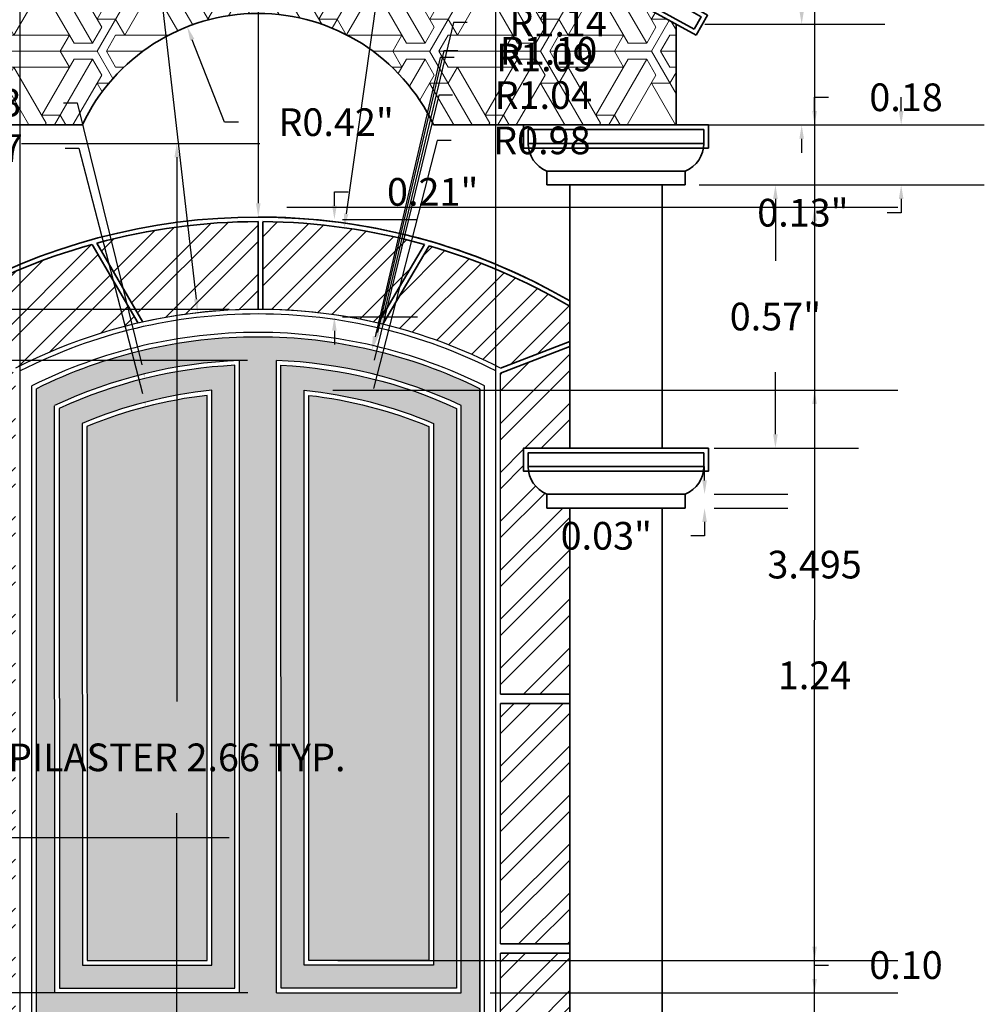
# Model space of a CAD drawing. Units: inches. Extents: x 19.36 to 24.97, y -1.46 to 4.09.
# Tile 3 of 4: x 20.47 to 22.56, y 0.85 to 2.98. Entities that reach past the tile are written whole.
import ezdxf

# ---------------------------------------------------------------- set-up
doc = ezdxf.new("R2010")
doc.units = ezdxf.units.IN
doc.header["$MEASUREMENT"] = 0
for name, color, linetype, lineweight in [('A-ANNO-DIMS', 2, 'Continuous', 18), ('A-COLS', 3, 'Continuous', 35), ('A-DOOR', 4, 'Continuous', 25), ('A-ELEV', 7, 'Continuous', 35), ('A-ELEV-PATT', 8, 'Continuous', 13)]:
    doc.layers.add(name, color=color, linetype=linetype, lineweight=lineweight)
doc.styles.get("Standard").update_dxf_attribs({"font": 'arial.ttf'})
doc.dimstyles.get("Standard").update_dxf_attribs({"dimtxt": 0.06, "dimasz": 0.03, "dimexe": 0.18, "dimexo": 0.0625, "dimgap": 0.09, "dimtad": 0, "dimtih": 1, "dimtoh": 1, "dimzin": 0, "dimdsep": 46, "dimlunit": 3, "dimtxsty": 'Standard', "dimcen": 0, "dimadec": 0, "dimazin": 0, "dimtfac": 1, "dimtofl": 0, "dimtmove": 0, "dimatfit": 3, "dimfxl": 1, "dimtolj": 1, "dimtzin": 0, "dimarcsym": 1})

# ---------------------------------------------------------------- blocks, each defined once
blk = doc.blocks.new('*D5')
at = {"layer": 'A-ANNO-DIMS', "color": 0, "lineweight": -2, "transparency": 16777216}
for p, q in [((21.1539, 2.5751), (21.1539, 2.6051)), ((21.1539, 2.6051), (21.1839, 2.6051)), ((21.1717, 2.5451), (21.3339, 2.5451)), ((21.1717, 2.3341), (21.3339, 2.3341)), ((21.1539, 2.3041), (21.1539, 2.2741))]:
    blk.add_line(p, q, dxfattribs=at)
at = {"layer": 'A-ANNO-DIMS', "color": 0, "transparency": 16777216}
for points in [[(21.1489, 2.5751), (21.1589, 2.5751), (21.1539, 2.5451)], [(21.1489, 2.3041), (21.1589, 2.3041), (21.1539, 2.3341)]]:
    blk.add_solid(points, dxfattribs=at)
at = {"layer": 'Defpoints', "color": 0, "transparency": 16777216}
for p in [(21.1092, 2.5451), (21.1539, 2.5451), (21.1092, 2.3341)]:
    blk.add_point(p, dxfattribs=at)
at = {"layer": 'A-ANNO-DIMS', "color": 0, "transparency": 16777216, "insert": (21.3667, 2.6051), "char_height": 0.06, "attachment_point": 5}
blk.add_mtext('\\A1;0.21"', dxfattribs=at)
blk = doc.blocks.new('*D6')
at = {"layer": 'A-ANNO-DIMS', "color": 0, "lineweight": -2, "transparency": 16777216}
for p, q in [((22.1656, 2.9981), (22.1656, 3.0281)), ((22.1656, 3.0281), (22.1956, 3.0281)), ((21.9561, 2.9681), (22.3456, 2.9681)), ((21.9561, 2.75), (22.3456, 2.75)), ((22.1656, 2.72), (22.1656, 2.69))]:
    blk.add_line(p, q, dxfattribs=at)
at = {"layer": 'A-ANNO-DIMS', "color": 0, "transparency": 16777216}
for points in [[(22.1606, 2.9981), (22.1706, 2.9981), (22.1656, 2.9681)], [(22.1606, 2.72), (22.1706, 2.72), (22.1656, 2.75)]]:
    blk.add_solid(points, dxfattribs=at)
at = {"layer": 'Defpoints', "color": 0, "transparency": 16777216}
for p in [(21.8936, 2.9681), (22.1656, 2.9681), (21.8936, 2.75)]:
    blk.add_point(p, dxfattribs=at)
at = {"layer": 'A-ANNO-DIMS', "color": 0, "transparency": 16777216, "insert": (22.3783, 3.0281), "char_height": 0.06, "attachment_point": 5}
blk.add_mtext('\\A1;0.22"', dxfattribs=at)
blk = doc.blocks.new('*D7')
at = {"layer": 'A-ANNO-DIMS', "color": 0, "lineweight": -2, "transparency": 16777216}
for p, q in [((22.381, 2.78), (22.381, 2.81)), ((21.9439, 2.75), (22.561, 2.75)), ((21.9439, 2.62), (22.561, 2.62)), ((22.381, 2.59), (22.381, 2.56)), ((22.381, 2.56), (22.351, 2.56))]:
    blk.add_line(p, q, dxfattribs=at)
at = {"layer": 'A-ANNO-DIMS', "color": 0, "transparency": 16777216}
for points in [[(22.376, 2.78), (22.386, 2.78), (22.381, 2.75)], [(22.376, 2.59), (22.386, 2.59), (22.381, 2.62)]]:
    blk.add_solid(points, dxfattribs=at)
at = {"layer": 'Defpoints', "color": 0, "transparency": 16777216}
for p in [(21.8814, 2.75), (21.8814, 2.62), (22.381, 2.62)]:
    blk.add_point(p, dxfattribs=at)
at = {"layer": 'A-ANNO-DIMS', "color": 0, "transparency": 16777216, "insert": (22.1683, 2.56), "char_height": 0.06, "attachment_point": 5}
blk.add_mtext('\\A1;0.13"', dxfattribs=at)
blk = doc.blocks.new('*D8')
at = {"layer": 'A-ANNO-DIMS', "color": 0, "lineweight": -2, "transparency": 16777216}
for p, q in [((21.9666, 2.62), (22.2888, 2.62)), ((22.1088, 2.59), (22.1088, 2.4556)), ((22.1088, 2.08), (22.1088, 2.2144)), ((21.9761, 2.05), (22.2888, 2.05))]:
    blk.add_line(p, q, dxfattribs=at)
at = {"layer": 'A-ANNO-DIMS', "color": 0, "transparency": 16777216}
for points in [[(22.1038, 2.59), (22.1138, 2.59), (22.1088, 2.62)], [(22.1038, 2.08), (22.1138, 2.08), (22.1088, 2.05)]]:
    blk.add_solid(points, dxfattribs=at)
at = {"layer": 'Defpoints', "color": 0, "transparency": 16777216}
for p in [(21.9041, 2.62), (21.9136, 2.05), (22.1088, 2.05)]:
    blk.add_point(p, dxfattribs=at)
at = {"layer": 'A-ANNO-DIMS', "color": 0, "transparency": 16777216, "insert": (22.1088, 2.335), "char_height": 0.06, "attachment_point": 5}
blk.add_mtext('\\A1;0.57"', dxfattribs=at)
blk = doc.blocks.new('*D9')
at = {"layer": 'A-ANNO-DIMS', "color": 0, "lineweight": -2, "transparency": 16777216}
for p, q in [((21.9554, 1.98), (21.9554, 2.01)), ((21.9761, 1.95), (22.1354, 1.95)), ((21.9761, 1.92), (22.1354, 1.92)), ((21.9554, 1.89), (21.9554, 1.86)), ((21.9554, 1.86), (21.9254, 1.86))]:
    blk.add_line(p, q, dxfattribs=at)
at = {"layer": 'A-ANNO-DIMS', "color": 0, "transparency": 16777216}
for points in [[(21.9504, 1.98), (21.9604, 1.98), (21.9554, 1.95)], [(21.9504, 1.89), (21.9604, 1.89), (21.9554, 1.92)]]:
    blk.add_solid(points, dxfattribs=at)
at = {"layer": 'Defpoints', "color": 0, "transparency": 16777216}
for p in [(21.9136, 1.95), (21.9136, 1.92), (21.9554, 1.92)]:
    blk.add_point(p, dxfattribs=at)
at = {"layer": 'A-ANNO-DIMS', "color": 0, "transparency": 16777216, "insert": (21.7426, 1.86), "char_height": 0.06, "attachment_point": 5}
blk.add_mtext('\\A1;0.03"', dxfattribs=at)
blk = doc.blocks.new('*D15')
at = {"layer": 'A-ANNO-DIMS', "color": 0, "lineweight": -2, "transparency": 16777216}
for p, q in [((20.9161, 2.7561), (20.8461, 2.9348)), ((20.9461, 2.7561), (20.9161, 2.7561))]:
    blk.add_line(p, q, dxfattribs=at)
at = {"layer": 'A-ANNO-DIMS', "color": 0, "transparency": 16777216}
blk.add_solid([(20.8507, 2.9366), (20.8414, 2.933), (20.8351, 2.9627)], dxfattribs=at)
at = {"layer": 'Defpoints', "color": 0, "transparency": 16777216}
for p in [(20.8351, 2.9627), (20.9884, 2.5717)]:
    blk.add_point(p, dxfattribs=at)
at = {"layer": 'A-ANNO-DIMS', "color": 0, "transparency": 16777216, "insert": (21.1576, 2.7561), "char_height": 0.06, "attachment_point": 5}
blk.add_mtext('\\A1;R0.42"', dxfattribs=at)
blk = doc.blocks.new('PILASTER')
for p, q in [((20.1136, 2.65), (20.0636, 2.65)), ((20.1136, 2.65), (20.0636, 2.65)), ((20.0636, 2.65), (20.0636, 2.62)), ((20.1136, 2.65), (20.3136, 2.65)), ((20.1136, 2.65), (20.3136, 2.65)), ((20.3136, 2.65), (20.3636, 2.65)), ((20.3136, 2.65), (20.3636, 2.65)), ((20.3636, 2.62), (20.3636, 2.65)), ((20.1136, 2.62), (20.0636, 2.62)), ((20.1136, 2.62), (20.0636, 2.62)), ((20.1136, 2.05), (20.1136, 2.62)), ((20.1136, 2.62), (20.3136, 2.62)), ((20.1136, 2.62), (20.3136, 2.62)), ((20.3136, 2.05), (20.3136, 2.62)), ((20.3136, 2.62), (20.3636, 2.62)), ((20.3136, 2.62), (20.3636, 2.62)), ((20.1136, 1.95), (20.0636, 1.95)), ((20.0636, 1.95), (20.0636, 1.92)), ((20.1136, 1.95), (20.3136, 1.95)), ((20.3136, 1.95), (20.3636, 1.95)), ((20.3636, 1.92), (20.3636, 1.95)), ((20.1136, 1.92), (20.0636, 1.92)), ((20.1136, 0.15), (20.1136, 1.92)), ((20.1136, 1.92), (20.3136, 1.92)), ((20.3136, 0.15), (20.3136, 1.92)), ((20.3136, 1.92), (20.3636, 1.92))]:
    blk.add_line(p, q)
for centre, start, end in [((20.0886, 2.71), 180, 247.3801), ((20.3386, 2.71), 292.6199, 0), ((20.0886, 2.01), 180, 247.3801), ((20.3386, 2.01), 292.6199, 0)]:
    blk.add_arc(centre, 0.065, start, end)
blk = doc.blocks.new('*D17')
at = {"layer": 'A-ANNO-DIMS', "color": 0, "lineweight": -2, "transparency": 16777216}
for p, q in [((20.4761, 2.71), (20.9926, 2.71)), ((20.8126, 2.68), (20.8126, 1.501)), ((20.8126, 0.08), (20.8126, 1.259)), ((20.4761, 0.05), (20.9926, 0.05))]:
    blk.add_line(p, q, dxfattribs=at)
at = {"layer": 'A-ANNO-DIMS', "color": 0, "transparency": 16777216}
for points in [[(20.8076, 2.68), (20.8176, 2.68), (20.8126, 2.71)], [(20.8076, 0.08), (20.8176, 0.08), (20.8126, 0.05)]]:
    blk.add_solid(points, dxfattribs=at)
at = {"layer": 'Defpoints', "color": 0, "transparency": 16777216}
for p in [(20.4136, 2.71), (20.8126, 2.71), (20.4136, 0.05)]:
    blk.add_point(p, dxfattribs=at)
at = {"layer": 'A-ANNO-DIMS', "color": 0, "transparency": 16777216, "insert": (20.8126, 1.38), "char_height": 0.06, "attachment_point": 5}
blk.add_mtext('\\A1;PILASTER 2.66 TYP.', dxfattribs=at)
blk = doc.blocks.new('*D20')
at = {"layer": 'A-ANNO-DIMS', "color": 0, "lineweight": -2, "transparency": 16777216}
for p, q in [((21.0509, 3.5451), (22.3736, 3.5451)), ((22.1936, 3.5151), (22.1936, 1.9182)), ((22.1936, 0.08), (22.1936, 1.6769)), ((22.0261, 0.05), (22.3736, 0.05))]:
    blk.add_line(p, q, dxfattribs=at)
at = {"layer": 'A-ANNO-DIMS', "color": 0, "transparency": 16777216}
for points in [[(22.1886, 3.5151), (22.1986, 3.5151), (22.1936, 3.5451)], [(22.1886, 0.08), (22.1986, 0.08), (22.1936, 0.05)]]:
    blk.add_solid(points, dxfattribs=at)
at = {"layer": 'Defpoints', "color": 0, "transparency": 16777216}
for p in [(20.9884, 3.5451), (22.1936, 3.5451), (21.9636, 0.05)]:
    blk.add_point(p, dxfattribs=at)
at = {"layer": 'A-ANNO-DIMS', "color": 0, "transparency": 16777216, "insert": (22.1936, 1.7976), "char_height": 0.06, "attachment_point": 5}
blk.add_mtext('\\A1;3.495', dxfattribs=at)
blk = doc.blocks.new('*D21')
at = {"layer": 'A-ANNO-DIMS', "color": 0, "lineweight": -2, "transparency": 16777216}
for p, q in [((20.4736, 0.1125), (20.4736, 4.0914)), ((21.5036, 0.1125), (21.5036, 4.0914)), ((20.5036, 3.9114), (20.8235, 3.9114)), ((21.4736, 3.9114), (21.1537, 3.9114))]:
    blk.add_line(p, q, dxfattribs=at)
at = {"layer": 'A-ANNO-DIMS', "color": 0, "transparency": 16777216}
for points in [[(20.5036, 3.9164), (20.5036, 3.9064), (20.4736, 3.9114)], [(21.4736, 3.9164), (21.4736, 3.9064), (21.5036, 3.9114)]]:
    blk.add_solid(points, dxfattribs=at)
at = {"layer": 'Defpoints', "color": 0, "transparency": 16777216}
for p in [(21.5036, 3.9114), (20.4736, 0.05), (21.5036, 0.05)]:
    blk.add_point(p, dxfattribs=at)
at = {"layer": 'A-ANNO-DIMS', "color": 0, "transparency": 16777216, "insert": (20.9886, 3.9114), "char_height": 0.06, "attachment_point": 5}
blk.add_mtext('\\A1;1.03', dxfattribs=at)
blk = doc.blocks.new('*D23')
at = {"layer": 'A-ANNO-DIMS', "color": 0, "lineweight": -2, "transparency": 16777216}
for p, q in [((20.9261, 1.2054), (19.3594, 1.2054)), ((19.5394, 1.1754), (19.5394, 0.7483)), ((19.5394, 0.08), (19.5394, 0.5071)), ((20.4111, 0.05), (19.3594, 0.05))]:
    blk.add_line(p, q, dxfattribs=at)
at = {"layer": 'A-ANNO-DIMS', "color": 0, "transparency": 16777216}
for points in [[(19.5344, 1.1754), (19.5444, 1.1754), (19.5394, 1.2054)], [(19.5344, 0.08), (19.5444, 0.08), (19.5394, 0.05)]]:
    blk.add_solid(points, dxfattribs=at)
at = {"layer": 'Defpoints', "color": 0, "transparency": 16777216}
for p in [(19.5394, 1.2054), (20.9886, 1.2054), (20.4736, 0.05)]:
    blk.add_point(p, dxfattribs=at)
at = {"layer": 'A-ANNO-DIMS', "color": 0, "transparency": 16777216, "insert": (19.5394, 0.6277), "char_height": 0.06, "attachment_point": 5}
blk.add_mtext('\\A1;1.16', dxfattribs=at)
blk = doc.blocks.new('*D24')
at = {"layer": 'A-ANNO-DIMS', "color": 0, "lineweight": -2, "transparency": 16777216}
for p, q in [((20.4089, 2.2147), (19.3594, 2.2147)), ((19.5394, 2.1847), (19.5394, 1.8307)), ((19.5394, 1.2354), (19.5394, 1.5894)), ((20.9261, 1.2054), (19.3594, 1.2054))]:
    blk.add_line(p, q, dxfattribs=at)
at = {"layer": 'A-ANNO-DIMS', "color": 0, "transparency": 16777216}
for points in [[(19.5344, 2.1847), (19.5444, 2.1847), (19.5394, 2.2147)], [(19.5344, 1.2354), (19.5444, 1.2354), (19.5394, 1.2054)]]:
    blk.add_solid(points, dxfattribs=at)
at = {"layer": 'Defpoints', "color": 0, "transparency": 16777216}
for p in [(19.5394, 2.2147), (20.4714, 2.2147), (20.9886, 1.2054)]:
    blk.add_point(p, dxfattribs=at)
at = {"layer": 'A-ANNO-DIMS', "color": 0, "transparency": 16777216, "insert": (19.5394, 1.71), "char_height": 0.06, "attachment_point": 5}
blk.add_mtext('\\A1;1.01', dxfattribs=at)
blk = doc.blocks.new('*D25')
at = {"layer": 'A-ANNO-DIMS', "color": 0, "lineweight": -2, "transparency": 16777216}
for p, q in [((19.5394, 2.3806), (19.5394, 2.4106)), ((19.5394, 2.4106), (19.5694, 2.4106)), ((20.9261, 2.3506), (19.3594, 2.3506)), ((20.4089, 2.2147), (19.3594, 2.2147)), ((19.5394, 2.1847), (19.5394, 2.1547))]:
    blk.add_line(p, q, dxfattribs=at)
at = {"layer": 'A-ANNO-DIMS', "color": 0, "transparency": 16777216}
for points in [[(19.5344, 2.3806), (19.5444, 2.3806), (19.5394, 2.3506)], [(19.5344, 2.1847), (19.5444, 2.1847), (19.5394, 2.2147)]]:
    blk.add_solid(points, dxfattribs=at)
at = {"layer": 'Defpoints', "color": 0, "transparency": 16777216}
for p in [(19.5394, 2.3506), (20.9886, 2.3506), (20.4714, 2.2147)]:
    blk.add_point(p, dxfattribs=at)
at = {"layer": 'A-ANNO-DIMS', "color": 0, "transparency": 16777216, "insert": (19.7372, 2.4106), "char_height": 0.06, "attachment_point": 5}
blk.add_mtext('\\A1;0.14', dxfattribs=at)
blk = doc.blocks.new('*D30')
at = {"layer": 'A-ANNO-DIMS', "color": 0, "lineweight": -2, "transparency": 16777216}
for p, q in [((22.1936, 0.9), (22.1936, 0.93)), ((22.1936, 0.93), (22.2236, 0.93)), ((21.4911, 0.87), (22.3736, 0.87)), ((21.4911, 0.77), (22.3736, 0.77)), ((22.1936, 0.74), (22.1936, 0.71))]:
    blk.add_line(p, q, dxfattribs=at)
at = {"layer": 'A-ANNO-DIMS', "color": 0, "transparency": 16777216}
for points in [[(22.1886, 0.9), (22.1986, 0.9), (22.1936, 0.87)], [(22.1886, 0.74), (22.1986, 0.74), (22.1936, 0.77)]]:
    blk.add_solid(points, dxfattribs=at)
at = {"layer": 'Defpoints', "color": 0, "transparency": 16777216}
for p in [(21.4286, 0.87), (22.1936, 0.87), (21.4286, 0.77)]:
    blk.add_point(p, dxfattribs=at)
at = {"layer": 'A-ANNO-DIMS', "color": 0, "transparency": 16777216, "insert": (22.3915, 0.93), "char_height": 0.06, "attachment_point": 5}
blk.add_mtext('\\A1;0.10', dxfattribs=at)
blk = doc.blocks.new('*D31')
at = {"layer": 'A-ANNO-DIMS', "color": 0, "lineweight": -2, "transparency": 16777216}
for p, q in [((20.9657, 2.2398), (19.3594, 2.2398)), ((19.5394, 2.2098), (19.5394, 1.6756)), ((19.5394, 0.9), (19.5394, 1.4342)), ((20.9661, 0.87), (19.3594, 0.87))]:
    blk.add_line(p, q, dxfattribs=at)
at = {"layer": 'A-ANNO-DIMS', "color": 0, "transparency": 16777216}
for points in [[(19.5344, 2.2098), (19.5444, 2.2098), (19.5394, 2.2398)], [(19.5344, 0.9), (19.5444, 0.9), (19.5394, 0.87)]]:
    blk.add_solid(points, dxfattribs=at)
at = {"layer": 'Defpoints', "color": 0, "transparency": 16777216}
for p in [(19.5394, 2.2398), (21.0282, 2.2398), (21.0286, 0.87)]:
    blk.add_point(p, dxfattribs=at)
at = {"layer": 'A-ANNO-DIMS', "color": 0, "transparency": 16777216, "insert": (19.5394, 1.5549), "char_height": 0.06, "attachment_point": 5}
blk.add_mtext('\\A1;1.37', dxfattribs=at)
blk = doc.blocks.new('*D33')
at = {"layer": 'A-ANNO-DIMS', "color": 0, "lineweight": -2, "transparency": 16777216}
for p, q in [((21.1507, 2.1755), (22.3736, 2.1755)), ((22.1936, 2.1455), (22.1936, 1.6779)), ((22.1936, 0.97), (22.1936, 1.4376)), ((21.1611, 0.94), (22.3736, 0.94))]:
    blk.add_line(p, q, dxfattribs=at)
at = {"layer": 'A-ANNO-DIMS', "color": 0, "transparency": 16777216}
for points in [[(22.1886, 2.1455), (22.1986, 2.1455), (22.1936, 2.1755)], [(22.1886, 0.97), (22.1986, 0.97), (22.1936, 0.94)]]:
    blk.add_solid(points, dxfattribs=at)
at = {"layer": 'Defpoints', "color": 0, "transparency": 16777216}
for p in [(21.0882, 2.1755), (22.1936, 2.1755), (21.0986, 0.94)]:
    blk.add_point(p, dxfattribs=at)
at = {"layer": 'A-ANNO-DIMS', "color": 0, "transparency": 16777216, "insert": (22.1936, 1.5577), "char_height": 0.06, "attachment_point": 5}
blk.add_mtext('\\A1;1.24', dxfattribs=at)
blk = doc.blocks.new('*D35')
at = {"layer": 'A-ANNO-DIMS', "color": 0, "lineweight": -2, "transparency": 16777216}
for p, q in [((22.1936, 2.78), (22.1936, 2.81)), ((22.1936, 2.81), (22.2236, 2.81)), ((21.4311, 2.75), (22.3736, 2.75)), ((21.0509, 2.5717), (22.3736, 2.5717)), ((22.1936, 2.5417), (22.1936, 2.5117))]:
    blk.add_line(p, q, dxfattribs=at)
at = {"layer": 'A-ANNO-DIMS', "color": 0, "transparency": 16777216}
for points in [[(22.1886, 2.78), (22.1986, 2.78), (22.1936, 2.75)], [(22.1886, 2.5417), (22.1986, 2.5417), (22.1936, 2.5717)]]:
    blk.add_solid(points, dxfattribs=at)
at = {"layer": 'Defpoints', "color": 0, "transparency": 16777216}
for p in [(21.3686, 2.75), (22.1936, 2.75), (20.9884, 2.5717)]:
    blk.add_point(p, dxfattribs=at)
at = {"layer": 'A-ANNO-DIMS', "color": 0, "transparency": 16777216, "insert": (22.3916, 2.81), "char_height": 0.06, "attachment_point": 5}
blk.add_mtext('\\A1;0.18', dxfattribs=at)
blk = doc.blocks.new('*D36')
at = {"layer": 'A-ANNO-DIMS', "color": 0, "lineweight": -2, "transparency": 16777216}
for p, q in [((20.9578, 3.2437), (20.9878, 3.2437)), ((20.9878, 3.2437), (20.988, 3.0217))]:
    blk.add_line(p, q, dxfattribs=at)
at = {"layer": 'A-ANNO-DIMS', "color": 0, "transparency": 16777216}
blk.add_solid([(20.993, 3.0217), (20.983, 3.0217), (20.988, 2.9917)], dxfattribs=at)
at = {"layer": 'Defpoints', "color": 0, "transparency": 16777216}
for p in [(20.988, 2.9917), (20.9884, 2.5717)]:
    blk.add_point(p, dxfattribs=at)
at = {"layer": 'A-ANNO-DIMS', "color": 0, "transparency": 16777216, "insert": (20.7614, 3.2437), "char_height": 0.06, "attachment_point": 5}
blk.add_mtext('\\A1;R0.42', dxfattribs=at)
blk = doc.blocks.new('*D37')
at = {"layer": 'A-ANNO-DIMS', "color": 0, "lineweight": -2, "transparency": 16777216}
for p, q in [((20.9892, 3.3577), (20.989, 2.5805)), ((21.0192, 3.3577), (20.9892, 3.3577))]:
    blk.add_line(p, q, dxfattribs=at)
at = {"layer": 'A-ANNO-DIMS', "color": 0, "transparency": 16777216}
blk.add_solid([(20.984, 2.5806), (20.994, 2.5805), (20.989, 2.5505)], dxfattribs=at)
at = {"layer": 'Defpoints', "color": 0, "transparency": 16777216}
for p in [(20.989, 2.5505), (20.9886, 1.2054)]:
    blk.add_point(p, dxfattribs=at)
at = {"layer": 'A-ANNO-DIMS', "color": 0, "transparency": 16777216, "insert": (21.2161, 3.3577), "char_height": 0.06, "attachment_point": 5}
blk.add_mtext('\\A1;R1.35', dxfattribs=at)
blk = doc.blocks.new('*D38')
at = {"layer": 'A-ANNO-DIMS', "color": 0, "lineweight": -2, "transparency": 16777216}
for p, q in [((21.2869, 3.3207), (21.1793, 2.5572)), ((21.3169, 3.3207), (21.2869, 3.3207))]:
    blk.add_line(p, q, dxfattribs=at)
at = {"layer": 'A-ANNO-DIMS', "color": 0, "transparency": 16777216}
blk.add_solid([(21.1743, 2.5579), (21.1842, 2.5565), (21.1751, 2.5275)], dxfattribs=at)
at = {"layer": 'Defpoints', "color": 0, "transparency": 16777216}
for p in [(21.1751, 2.5275), (20.9886, 1.2054)]:
    blk.add_point(p, dxfattribs=at)
at = {"layer": 'A-ANNO-DIMS', "color": 0, "transparency": 16777216, "insert": (21.5134, 3.3207), "char_height": 0.06, "attachment_point": 5}
blk.add_mtext('\\A1;R1.34', dxfattribs=at)
blk = doc.blocks.new('*D39')
at = {"layer": 'A-ANNO-DIMS', "color": 0, "lineweight": -2, "transparency": 16777216}
for p, q in [((20.7496, 3.0257), (20.7796, 3.0257)), ((20.7796, 3.0257), (20.8546, 2.3729))]:
    blk.add_line(p, q, dxfattribs=at)
at = {"layer": 'A-ANNO-DIMS', "color": 0, "transparency": 16777216}
blk.add_solid([(20.8595, 2.3734), (20.8496, 2.3723), (20.858, 2.3431)], dxfattribs=at)
at = {"layer": 'Defpoints', "color": 0, "transparency": 16777216}
for p in [(20.858, 2.3431), (20.9886, 1.2054)]:
    blk.add_point(p, dxfattribs=at)
at = {"layer": 'A-ANNO-DIMS', "color": 0, "transparency": 16777216, "insert": (20.5527, 3.0257), "char_height": 0.06, "attachment_point": 5}
blk.add_mtext('\\A1;R1.15', dxfattribs=at)
blk = doc.blocks.new('*D40')
at = {"layer": 'A-ANNO-DIMS', "color": 0, "lineweight": -2, "transparency": 16777216}
for p, q in [((21.4117, 2.9717), (21.2601, 2.3385)), ((21.4417, 2.9717), (21.4117, 2.9717))]:
    blk.add_line(p, q, dxfattribs=at)
at = {"layer": 'A-ANNO-DIMS', "color": 0, "transparency": 16777216}
blk.add_solid([(21.2552, 2.3397), (21.2649, 2.3373), (21.2531, 2.3093)], dxfattribs=at)
at = {"layer": 'Defpoints', "color": 0, "transparency": 16777216}
for p in [(21.2531, 2.3093), (20.9886, 1.2054)]:
    blk.add_point(p, dxfattribs=at)
at = {"layer": 'A-ANNO-DIMS', "color": 0, "transparency": 16777216, "insert": (21.6383, 2.9717), "char_height": 0.06, "attachment_point": 5}
blk.add_mtext('\\A1;R1.14', dxfattribs=at)
blk = doc.blocks.new('*D41')
at = {"layer": 'A-ANNO-DIMS', "color": 0, "lineweight": -2, "transparency": 16777216}
for p, q in [((21.3909, 2.9109), (21.247, 2.3005)), ((21.4209, 2.9109), (21.3909, 2.9109))]:
    blk.add_line(p, q, dxfattribs=at)
at = {"layer": 'A-ANNO-DIMS', "color": 0, "transparency": 16777216}
blk.add_solid([(21.2421, 2.3016), (21.2518, 2.2993), (21.2401, 2.2713)], dxfattribs=at)
at = {"layer": 'Defpoints', "color": 0, "transparency": 16777216}
for p in [(21.2401, 2.2713), (20.9886, 1.2054)]:
    blk.add_point(p, dxfattribs=at)
at = {"layer": 'A-ANNO-DIMS', "color": 0, "transparency": 16777216, "insert": (21.6175, 2.9109), "char_height": 0.06, "attachment_point": 5}
blk.add_mtext('\\A1;R1.10', dxfattribs=at)
blk = doc.blocks.new('*D42')
at = {"layer": 'A-ANNO-DIMS', "color": 0, "lineweight": -2, "transparency": 16777216}
for p, q in [((21.3829, 2.8963), (21.2419, 2.2914)), ((21.4129, 2.8963), (21.3829, 2.8963))]:
    blk.add_line(p, q, dxfattribs=at)
at = {"layer": 'A-ANNO-DIMS', "color": 0, "transparency": 16777216}
blk.add_solid([(21.237, 2.2926), (21.2467, 2.2903), (21.235, 2.2622)], dxfattribs=at)
at = {"layer": 'Defpoints', "color": 0, "transparency": 16777216}
for p in [(21.235, 2.2622), (20.9886, 1.2054)]:
    blk.add_point(p, dxfattribs=at)
at = {"layer": 'A-ANNO-DIMS', "color": 0, "transparency": 16777216, "insert": (21.6096, 2.8963), "char_height": 0.06, "attachment_point": 5}
blk.add_mtext('\\A1;R1.09', dxfattribs=at)
blk = doc.blocks.new('*D43')
at = {"layer": 'A-ANNO-DIMS', "color": 0, "lineweight": -2, "transparency": 16777216}
for p, q in [((21.3797, 2.8148), (21.2402, 2.2404)), ((21.4097, 2.8148), (21.3797, 2.8148))]:
    blk.add_line(p, q, dxfattribs=at)
at = {"layer": 'A-ANNO-DIMS', "color": 0, "transparency": 16777216}
blk.add_solid([(21.2353, 2.2416), (21.245, 2.2392), (21.2331, 2.2113)], dxfattribs=at)
at = {"layer": 'Defpoints', "color": 0, "transparency": 16777216}
for p in [(21.2331, 2.2113), (20.9886, 1.2054)]:
    blk.add_point(p, dxfattribs=at)
at = {"layer": 'A-ANNO-DIMS', "color": 0, "transparency": 16777216, "insert": (21.6062, 2.8148), "char_height": 0.06, "attachment_point": 5}
blk.add_mtext('\\A1;R1.04', dxfattribs=at)
blk = doc.blocks.new('*D44')
at = {"layer": 'A-ANNO-DIMS', "color": 0, "lineweight": -2, "transparency": 16777216}
for p, q in [((20.5672, 2.7983), (20.5972, 2.7983)), ((20.5972, 2.7983), (20.7369, 2.2301))]:
    blk.add_line(p, q, dxfattribs=at)
at = {"layer": 'A-ANNO-DIMS', "color": 0, "transparency": 16777216}
blk.add_solid([(20.7417, 2.2313), (20.732, 2.2289), (20.744, 2.2009)], dxfattribs=at)
at = {"layer": 'Defpoints', "color": 0, "transparency": 16777216}
for p in [(20.744, 2.2009), (20.9886, 1.2054)]:
    blk.add_point(p, dxfattribs=at)
at = {"layer": 'A-ANNO-DIMS', "color": 0, "transparency": 16777216, "insert": (20.3706, 2.7983), "char_height": 0.06, "attachment_point": 5}
blk.add_mtext('\\A1;R1.03', dxfattribs=at)
blk = doc.blocks.new('*D45')
at = {"layer": 'A-ANNO-DIMS', "color": 0, "lineweight": -2, "transparency": 16777216}
for p, q in [((21.3764, 2.7167), (21.2384, 2.179)), ((21.4064, 2.7167), (21.3764, 2.7167))]:
    blk.add_line(p, q, dxfattribs=at)
at = {"layer": 'A-ANNO-DIMS', "color": 0, "transparency": 16777216}
blk.add_solid([(21.2336, 2.1803), (21.2433, 2.1778), (21.231, 2.15)], dxfattribs=at)
at = {"layer": 'Defpoints', "color": 0, "transparency": 16777216}
for p in [(21.231, 2.15), (20.9886, 1.2054)]:
    blk.add_point(p, dxfattribs=at)
at = {"layer": 'A-ANNO-DIMS', "color": 0, "transparency": 16777216, "insert": (21.6031, 2.7167), "char_height": 0.06, "attachment_point": 5}
blk.add_mtext('\\A1;R0.98', dxfattribs=at)
blk = doc.blocks.new('*D46')
at = {"layer": 'A-ANNO-DIMS', "color": 0, "lineweight": -2, "transparency": 16777216}
for p, q in [((20.5706, 2.7001), (20.6006, 2.7001)), ((20.6006, 2.7001), (20.7386, 2.1686))]:
    blk.add_line(p, q, dxfattribs=at)
at = {"layer": 'A-ANNO-DIMS', "color": 0, "transparency": 16777216}
blk.add_solid([(20.7434, 2.1699), (20.7337, 2.1674), (20.7461, 2.1396)], dxfattribs=at)
at = {"layer": 'Defpoints', "color": 0, "transparency": 16777216}
for p in [(20.7461, 2.1396), (20.9886, 1.2054)]:
    blk.add_point(p, dxfattribs=at)
at = {"layer": 'A-ANNO-DIMS', "color": 0, "transparency": 16777216, "insert": (20.374, 2.7001), "char_height": 0.06, "attachment_point": 5}
blk.add_mtext('\\A1;R0.97', dxfattribs=at)

msp = doc.modelspace()

# ---------------------------------------------------------------- hatches: boundary and pattern name
at = {"layer": 'A-ELEV-PATT'}
h = msp.add_hatch(dxfattribs=at)
h.set_pattern_fill('ESCHER', color=256, scale=0.2)
h.paths.add_polyline_path([(20.9884, 3.4642), (20.0836, 2.9685), (20.0836, 2.75), (20.1136, 2.75), (20.3136, 2.75), (20.3636, 2.75), (20.4136, 2.75), (20.6081, 2.75, -0.635528), (21.3686, 2.75), (21.5636, 2.75), (21.6136, 2.75), (21.6636, 2.75), (21.8636, 2.75), (21.8936, 2.75), (21.8936, 2.9682)])
h = msp.add_hatch(dxfattribs=at)
h.set_pattern_fill('ANSI32', color=256, scale=0.2)
h.paths.add_polyline_path([(20.6294, 2.4913, 0.064491), (20.3136, 2.3574), (20.3136, 2.2989), (20.4636, 2.2231, -0.061889), (20.7287, 2.3207)])
h.paths.add_polyline_path([(20.9886, 2.5406, 0.066262), (20.6394, 2.4941), (20.7389, 2.323, -0.055018), (20.9886, 2.3506)])
h.paths.add_polyline_path([(21.3488, 2.491, 0.066519), (20.9986, 2.5405), (20.9986, 2.3505, -0.055118), (21.2486, 2.3207)])
h.paths.add_polyline_path([(21.6636, 2.3574, 0.062356), (21.3588, 2.4882), (21.2588, 2.3182, -0.0596), (21.5136, 2.2231), (21.6636, 2.2812)])
h.paths.add_polyline_path([(21.6636, 2.2704), (21.5136, 2.2124), (21.5136, 2.1846), (21.5136, 1.5166), (21.6636, 1.5166), (21.6636, 1.92), (21.6136, 1.92), (21.6136, 1.95, -0.261087), (21.5744, 2), (21.5636, 2), (21.5636, 2.05), (21.6136, 2.05), (21.6636, 2.05)])
h.paths.add_polyline_path([(21.6636, 1.4966), (21.5136, 1.4966), (21.5136, 0.9758), (21.6636, 0.9758)])
h.paths.add_polyline_path([(21.6636, 0.9558), (21.5136, 0.9558), (21.5136, 0.455), (21.6636, 0.455)])
h.paths.add_polyline_path([(21.6636, 0.435), (21.5136, 0.435), (21.5136, 0.08), (21.5636, 0.08), (21.5636, 0.1), (21.6136, 0.1), (21.6136, 0.15), (21.6636, 0.15)])
h.paths.add_polyline_path([(20.4636, 0.435), (20.3136, 0.435), (20.3136, 0.15), (20.3636, 0.15), (20.3636, 0.1), (20.4136, 0.1), (20.4136, 0.08), (20.4636, 0.08)])
h.paths.add_polyline_path([(20.4636, 0.9558), (20.3136, 0.9558), (20.3136, 0.455), (20.4636, 0.455)])
h.paths.add_polyline_path([(20.4636, 1.4966), (20.3136, 1.4966), (20.3136, 0.9758), (20.4636, 0.9758)])
h.paths.add_polyline_path([(20.4636, 2.1846), (20.4636, 2.2119), (20.3136, 2.2877), (20.3136, 2.05), (20.3636, 2.05), (20.4136, 2.05), (20.4136, 2), (20.4029, 2, -0.261087), (20.3636, 1.95), (20.3636, 1.92), (20.3136, 1.92), (20.3136, 1.5166), (20.4636, 1.5166)])
h = msp.add_hatch(color=256, dxfattribs=at)
h.dxf.hatch_style = 1
h.paths.add_polyline_path([(21.3586, 2.0968, 0.070017), (21.0982, 2.1643), (21.0986, 0.94), (21.3586, 0.94)], flags=0)
h.paths.add_polyline_path([(20.8785, 2.1642, 0.070014), (20.6181, 2.0966), (20.6186, 0.94), (20.8786, 0.94)], flags=0)
h.paths.add_polyline_path([(21.4686, 2.1786, 0.115049), (20.9886, 2.2906, 0.115049), (20.5086, 2.1786), (20.5086, 0.06), (20.8541, 0.06), (20.9886, 0.06), (21.1231, 0.06), (21.4686, 0.06)])
h.paths.add_polyline_path([(21.0282, 2.2398, -0.100527), (21.4286, 2.1424), (21.4286, 0.87), (21.0286, 0.87)], flags=16)
h.paths.add_polyline_path([(21.0382, 2.2294, -0.096406), (21.4186, 2.136), (21.4186, 0.88), (21.0386, 0.88)], flags=0)
h.paths.add_polyline_path([(20.9486, 0.87), (20.5484, 0.87), (20.5476, 2.1419, -0.10066), (20.9485, 2.2398)], flags=16)
h.paths.add_polyline_path([(20.9386, 0.88), (20.5586, 0.88), (20.5581, 2.1358, -0.096404), (20.9385, 2.2293)], flags=0)
h.paths.add_polyline_path([(21.0882, 2.1755, -0.074627), (21.3686, 2.1035), (21.3686, 0.93), (21.0886, 0.93)], flags=0)
h.paths.add_polyline_path([(21.0982, 2.1643, -0.070017), (21.3586, 2.0968), (21.3586, 0.94), (21.0986, 0.94)], flags=0)
h.paths.add_polyline_path([(20.8886, 0.93), (20.6086, 0.93), (20.6081, 2.1032, -0.074624), (20.8885, 2.1754)], flags=0)
h.paths.add_polyline_path([(20.8786, 0.94), (20.6186, 0.94), (20.6181, 2.0966, -0.070014), (20.8785, 2.1642)], flags=0)
h.paths.add_polyline_path([(21.0286, 0.77), (21.4286, 0.77), (21.4286, 0.1), (21.0286, 0.1)], flags=16)
h.paths.add_polyline_path([(20.9486, 0.77), (20.9486, 0.1), (20.5486, 0.1), (20.5486, 0.77)], flags=16)
h.paths.add_polyline_path([(21.0386, 0.76), (21.4186, 0.76), (21.4186, 0.11), (21.0386, 0.11)], flags=0)
h.paths.add_polyline_path([(20.9386, 0.76), (20.9386, 0.11), (20.5586, 0.11), (20.5586, 0.76)], flags=0)
h.paths.add_polyline_path([(21.0886, 0.71), (21.3686, 0.71), (21.3686, 0.16), (21.0886, 0.16)], flags=0)
h.paths.add_polyline_path([(20.8886, 0.71), (20.8886, 0.16), (20.6086, 0.16), (20.6086, 0.71)], flags=0)
h.paths.add_polyline_path([(21.0986, 0.7), (21.3586, 0.7), (21.3586, 0.17), (21.0986, 0.17)], flags=0)
h.paths.add_polyline_path([(20.8786, 0.7), (20.8786, 0.17), (20.6186, 0.17), (20.6186, 0.7)], flags=0)
h.paths.add_polyline_path([(21.3586, 0.7), (21.0986, 0.7), (21.0986, 0.17), (21.3586, 0.17)], flags=0)
h = msp.add_hatch(color=256, dxfattribs=at)
h.dxf.hatch_style = 1
h.paths.add_polyline_path([(20.8785, 2.1642, 0.070014), (20.6181, 2.0966), (20.6186, 0.94), (20.8786, 0.94)], flags=0)
h.paths.add_polyline_path([(20.9385, 2.2293, 0.096404), (20.5581, 2.1358), (20.5586, 0.88), (20.9386, 0.88)])
h.paths.add_polyline_path([(20.6086, 0.93), (20.8886, 0.93), (20.8885, 2.1754, 0.074624), (20.6081, 2.1032)], flags=16)
h.paths.add_polyline_path([(20.6181, 2.0966, -0.070014), (20.8785, 2.1642), (20.8786, 0.94), (20.6186, 0.94)], flags=0)
h.paths.add_polyline_path([(21.4186, 2.136, 0.096406), (21.0382, 2.2294), (21.0386, 0.88), (21.4186, 0.88)])
h.paths.add_polyline_path([(21.0882, 2.1755, -0.074627), (21.3686, 2.1035), (21.3686, 0.93), (21.0886, 0.93)], flags=16)
h.paths.add_polyline_path([(21.0982, 2.1643, -0.070017), (21.3586, 2.0968), (21.3586, 0.94), (21.0986, 0.94)], flags=0)
h.paths.add_polyline_path([(21.4186, 0.76), (21.0386, 0.76), (21.0386, 0.11), (21.4186, 0.11)])
h.paths.add_polyline_path([(21.0886, 0.71), (21.3686, 0.71), (21.3686, 0.16), (21.0886, 0.16)], flags=16)
h.paths.add_polyline_path([(21.0986, 0.7), (21.3586, 0.7), (21.3586, 0.17), (21.0986, 0.17)], flags=0)
h.paths.add_polyline_path([(20.9386, 0.76), (20.5586, 0.76), (20.5586, 0.11), (20.9386, 0.11)])
h.paths.add_polyline_path([(20.8886, 0.16), (20.6086, 0.16), (20.6086, 0.71), (20.8886, 0.71)], flags=16)
h.paths.add_polyline_path([(20.8786, 0.17), (20.6186, 0.17), (20.6186, 0.7), (20.8786, 0.7)], flags=0)
h = msp.add_hatch(color=256, dxfattribs=at)
h.dxf.hatch_style = 1
h.paths.add_polyline_path([(21.3586, 2.0968, 0.070017), (21.0982, 2.1643), (21.0986, 0.94), (21.3586, 0.94)])
h.paths.add_polyline_path([(21.3586, 0.7), (21.0986, 0.7), (21.0986, 0.17), (21.3586, 0.17)])
h.paths.add_polyline_path([(20.8785, 2.1642, 0.070014), (20.6181, 2.0966), (20.6186, 0.94), (20.8786, 0.94)])
h.paths.add_polyline_path([(20.8786, 0.7), (20.6186, 0.7), (20.6186, 0.17), (20.8786, 0.17)])

# ---------------------------------------------------------------- linework, layer by layer
at = {"layer": 'A-DOOR'}
for p, q in [((20.4736, 2.1913), (20.4738, 2.2171)), ((21.5036, 2.1913), (21.5036, 2.217)), ((21.5136, 2.1846), (21.5136, 2.2124)), ((20.8886, 0.93), (20.8885, 2.1754)), ((20.5484, 0.87), (20.5476, 2.1419)), ((20.6081, 2.1032), (20.6086, 0.93)), ((20.6086, 0.93), (20.8886, 0.93)), ((20.9486, 0.87), (20.5484, 0.87)), ((21.0286, 0.87), (21.4286, 0.87))]:
    msp.add_line(p, q, dxfattribs=at)
for points in [[(20.9486, 0.87), (20.9485, 2.2398)], [(21.0286, 0.87), (21.0282, 2.2398)], [(20.4736, 0.05), (20.4736, 2.1913)], [(20.4986, 0.05), (20.4986, 2.1848)], [(20.5086, 0.06), (20.5086, 2.1786)], [(21.4686, 2.1786), (21.4686, 0.06), (20.5086, 0.06)], [(21.4686, 0.06), (21.4686, 2.1786)], [(21.4786, 0.05), (21.4786, 2.1848)], [(21.5036, 0.05), (21.5036, 2.1913)], [(21.5136, 1.5166), (21.5136, 2.1846)], [(21.4286, 0.87), (21.4286, 2.1424)], [(21.5136, 0.9758), (21.5136, 1.4966)], [(21.5136, 0.455), (21.5136, 0.9558)], [(20.9486, 0.88), (20.9486, 0.88)], [(20.9386, 0.87), (20.9386, 0.87)]]:
    msp.add_lwpolyline(points, dxfattribs=at)
for points in [[(20.9386, 0.88), (20.9385, 2.2293, 0.096404), (20.5581, 2.1358), (20.5586, 0.88)], [(21.0386, 0.88), (21.0382, 2.2294, -0.096406), (21.4186, 2.136), (21.4186, 0.88)], [(20.8786, 0.94), (20.8785, 2.1642, 0.070014), (20.6181, 2.0966), (20.6186, 0.94)], [(21.0886, 0.93), (21.0882, 2.1755, -0.074627), (21.3686, 2.1035), (21.3686, 0.93)], [(21.0986, 0.94), (21.0982, 2.1643, -0.070017), (21.3586, 2.0968), (21.3586, 0.94)]]:
    msp.add_lwpolyline(points, format="xyb", close=True, dxfattribs=at)
for radius, start, end in [(1.1452, 76.8803, 117.2863), (1.1452, 90, 103.1205), (1.1452, 62.7137, 90), (1.1352, 90, 116.9703), (1.1352, 63.0208, 90), (1.0952, 90, 116.5776), (1.0852, 90, 116.2518), (1.0952, 63.4224, 90), (1.0852, 63.7482, 90), (1.0352, 92.2244, 115.2164), (1.0352, 64.8467, 87.8088), (0.9752, 95.8957, 112.9667)]:
    msp.add_arc((20.9886, 1.2054), radius, start, end, dxfattribs=at)
at = {"layer": 'A-ELEV'}
for p, q in [((21.8936, 2.75), (21.8936, 2.9681)), ((21.9636, 2.75), (21.9136, 2.75)), ((20.9886, 2.5406), (20.9886, 2.3506)), ((20.9986, 2.5505), (20.9986, 2.5505)), ((20.9986, 2.5405), (20.9986, 2.3506)), ((20.7287, 2.3207), (20.6294, 2.4913)), ((20.7389, 2.323), (20.6394, 2.4941)), ((21.2486, 2.3207), (21.3488, 2.491)), ((21.2588, 2.3182), (21.3588, 2.4882)), ((21.5136, 2.2231), (21.6636, 2.2812)), ((21.5136, 2.2124), (21.6636, 2.2704)), ((21.5136, 1.5166), (21.6636, 1.5166)), ((21.5136, 1.4966), (21.6636, 1.4966)), ((21.5136, 0.9758), (21.6636, 0.9758)), ((21.5136, 0.9558), (21.6636, 0.9558))]:
    msp.add_line(p, q, dxfattribs=at)
for points in [[(21.937, 2.9444), (21.962, 2.9877), (20.9884, 3.5451), (20.0148, 2.9877), (20.0398, 2.9444), (20.9884, 3.4642)], [(21.9332, 2.9579), (21.9483, 2.9841), (20.9884, 3.5336), (20.0285, 2.9841), (20.0436, 2.9579), (20.9884, 3.4756)], [(21.9636, 2.75), (21.9136, 2.75), (21.8636, 2.75), (21.6636, 2.75), (21.6136, 2.75), (21.5636, 2.75), (21.5636, 2.7), (21.6136, 2.7), (21.6636, 2.7), (21.8636, 2.7), (21.9136, 2.7), (21.9636, 2.7)], [(21.9536, 2.74), (21.9136, 2.74), (21.8636, 2.74), (21.6636, 2.74), (21.6136, 2.74), (21.5736, 2.74), (21.5736, 2.71), (21.6136, 2.71), (21.6636, 2.71), (21.8636, 2.71), (21.9136, 2.71), (21.9536, 2.71)], [(21.9636, 2.05), (21.9136, 2.05), (21.8636, 2.05), (21.6636, 2.05), (21.6136, 2.05), (21.5636, 2.05), (21.5636, 2), (21.6136, 2), (21.6636, 2), (21.8636, 2), (21.9136, 2), (21.9636, 2)], [(21.9536, 2.04), (21.9136, 2.04), (21.8636, 2.04), (21.6636, 2.04), (21.6136, 2.04), (21.5736, 2.04), (21.5736, 2.01), (21.6136, 2.01), (21.6636, 2.01), (21.8636, 2.01), (21.9136, 2.01), (21.9536, 2.01)]]:
    msp.add_lwpolyline(points, close=True, dxfattribs=at)
for points in [[(20.4136, 2.75), (20.6081, 2.75)], [(21.5636, 2.75), (21.3686, 2.75)]]:
    msp.add_lwpolyline(points, dxfattribs=at)
for centre, radius, start, end in [((20.9884, 2.5717), 0.42, 25.1258, 154.8742), ((20.9886, 1.2054), 1.3452, 59.8817, 120.1183), ((20.9886, 1.2054), 1.3352, 90, 105.1639), ((20.9886, 1.2054), 1.3352, 90, 105.1639), ((20.9886, 1.2054), 1.3452, 62.7137, 90), ((20.9886, 1.2054), 1.3352, 74.3483, 89.5709), ((20.9886, 1.2054), 1.3352, 74.3483, 89.5709), ((20.9886, 1.2054), 1.3352, 105.6078, 120.3675), ((20.9886, 1.2054), 1.3352, 59.6325, 73.9049)]:
    msp.add_arc(centre, radius, start, end, dxfattribs=at)

# ---------------------------------------------------------------- block references
at = {"layer": 'A-COLS', "extrusion": (0, 0, -1), "zscale": -1}
msp.add_blockref('PILASTER', (-41.9773, 0), dxfattribs=at)

# ---------------------------------------------------------------- dimensions: what is measured, and where the dimension line sits
at = {"layer": 'A-ANNO-DIMS'}
dim = msp.add_linear_dim(base=(21.5036, 3.9114), p1=(20.4736, 0.05), p2=(21.5036, 0.05), dimstyle='Standard', override={"dimdec": 2, "dimlfac": 1, "dimrnd": 0, "dimzin": 0, "dimdsep": 46, "dimlunit": 2}, dxfattribs=at)
dim.commit()
dim.dimension.update_dxf_attribs({"geometry": '*D21', "text_midpoint": (20.9886, 3.9114)})
for base, p1, p2, override, picture, middle in [((22.1936, 3.5451), (21.9636, 0.05), (20.9884, 3.5451), {"dimdec": 3, "dimlfac": 1, "dimrnd": 0, "dimzin": 0, "dimdsep": 46, "dimlunit": 2}, '*D20', (22.1936, 1.7976)), ((22.1656, 2.9681), (21.8936, 2.75), (21.8936, 2.9681), {"dimclrd": 0, "dimclre": 0, "dimclrt": 0}, '*D6', (22.3783, 3.0281)), ((22.1936, 2.75), (20.9884, 2.5717), (21.3686, 2.75), {"dimdec": 2, "dimlfac": 1, "dimrnd": 0, "dimzin": 0, "dimdsep": 46, "dimlunit": 2}, '*D35', (22.3916, 2.81)), ((22.381, 2.62), (21.8814, 2.75), (21.8814, 2.62), {"dimclrd": 0, "dimclre": 0, "dimclrt": 0}, '*D7', (22.1683, 2.56)), ((21.1539, 2.5451), (21.1092, 2.3341), (21.1092, 2.5451), {"dimclrd": 0, "dimclre": 0, "dimclrt": 0}, '*D5', (21.3667, 2.6051)), ((22.1088, 2.05), (21.9041, 2.62), (21.9136, 2.05), {"dimclrd": 0, "dimclre": 0, "dimclrt": 0}, '*D8', (22.1088, 2.335)), ((19.5394, 2.3506), (20.4714, 2.2147), (20.9886, 2.3506), {"dimdec": 2, "dimlfac": 1, "dimrnd": 0, "dimzin": 0, "dimdsep": 46, "dimlunit": 2}, '*D25', (19.7372, 2.4106)), ((19.5394, 2.2398), (21.0286, 0.87), (21.0282, 2.2398), {"dimdec": 2, "dimlfac": 1, "dimrnd": 0, "dimzin": 0, "dimdsep": 46, "dimlunit": 2}, '*D31', (19.5394, 1.5549)), ((19.5394, 2.2147), (20.9886, 1.2054), (20.4714, 2.2147), {"dimdec": 2, "dimlfac": 1, "dimrnd": 0, "dimzin": 0, "dimdsep": 46, "dimlunit": 2}, '*D24', (19.5394, 1.71)), ((22.1936, 2.1755), (21.0986, 0.94), (21.0882, 2.1755), {"dimdec": 2, "dimlfac": 1, "dimrnd": 0, "dimzin": 0, "dimdsep": 46, "dimlunit": 2}, '*D33', (22.1936, 1.5577)), ((21.9554, 1.92), (21.9136, 1.95), (21.9136, 1.92), {"dimclrd": 0, "dimclre": 0, "dimclrt": 0}, '*D9', (21.7426, 1.86)), ((19.5394, 1.2054), (20.4736, 0.05), (20.9886, 1.2054), {"dimdec": 2, "dimlfac": 1, "dimrnd": 0, "dimzin": 0, "dimdsep": 46, "dimlunit": 2}, '*D23', (19.5394, 0.6277)), ((22.1936, 0.87), (21.4286, 0.77), (21.4286, 0.87), {"dimdec": 2, "dimlfac": 1, "dimrnd": 0, "dimzin": 0, "dimdsep": 46, "dimlunit": 2}, '*D30', (22.3915, 0.93))]:
    dim = msp.add_linear_dim(base=base, p1=p1, p2=p2, angle=90, dimstyle='Standard', override=override, dxfattribs=at)
    dim.commit()
    dim.dimension.update_dxf_attribs({"geometry": picture, "text_midpoint": middle})
for center, mpoint, override, picture, middle in [((20.9886, 1.2054), (20.989, 2.5505), {"dimdec": 2, "dimlfac": 1, "dimrnd": 0, "dimzin": 0, "dimdsep": 46, "dimlunit": 2}, '*D37', (21.2161, 3.3577)), ((20.9886, 1.2054), (21.1751, 2.5275), {"dimdec": 2, "dimlfac": 1, "dimrnd": 0, "dimzin": 0, "dimdsep": 46, "dimlunit": 2}, '*D38', (21.5134, 3.3207)), ((20.9884, 2.5717), (20.988, 2.9917), {"dimdec": 2, "dimlfac": 1, "dimrnd": 0, "dimzin": 0, "dimdsep": 46, "dimlunit": 2}, '*D36', (20.7614, 3.2437)), ((20.9886, 1.2054), (20.858, 2.3431), {"dimdec": 2, "dimlfac": 1, "dimrnd": 0, "dimzin": 0, "dimdsep": 46, "dimlunit": 2}, '*D39', (20.5527, 3.0257)), ((20.9886, 1.2054), (21.2531, 2.3093), {"dimdec": 2, "dimlfac": 1, "dimrnd": 0, "dimzin": 0, "dimdsep": 46, "dimlunit": 2}, '*D40', (21.6383, 2.9717)), ((20.9884, 2.5717), (20.8351, 2.9627), {"dimclrd": 0, "dimclre": 0, "dimclrt": 0}, '*D15', (21.1576, 2.7561)), ((20.9886, 1.2054), (21.2401, 2.2713), {"dimdec": 2, "dimlfac": 1, "dimrnd": 0, "dimzin": 0, "dimdsep": 46, "dimlunit": 2}, '*D41', (21.6175, 2.9109)), ((20.9886, 1.2054), (21.235, 2.2622), {"dimdec": 2, "dimlfac": 1, "dimrnd": 0, "dimzin": 0, "dimdsep": 46, "dimlunit": 2}, '*D42', (21.6096, 2.8963)), ((20.9886, 1.2054), (20.744, 2.2009), {"dimdec": 2, "dimlfac": 1, "dimrnd": 0, "dimzin": 0, "dimdsep": 46, "dimlunit": 2}, '*D44', (20.3706, 2.7983)), ((20.9886, 1.2054), (21.2331, 2.2113), {"dimdec": 2, "dimlfac": 1, "dimrnd": 0, "dimzin": 0, "dimdsep": 46, "dimlunit": 2}, '*D43', (21.6062, 2.8148)), ((20.9886, 1.2054), (21.231, 2.15), {"dimdec": 2, "dimlfac": 1, "dimrnd": 0, "dimzin": 0, "dimdsep": 46, "dimlunit": 2}, '*D45', (21.6031, 2.7167)), ((20.9886, 1.2054), (20.7461, 2.1396), {"dimdec": 2, "dimlfac": 1, "dimrnd": 0, "dimzin": 0, "dimdsep": 46, "dimlunit": 2}, '*D46', (20.374, 2.7001))]:
    dim = msp.add_radius_dim(center=center, mpoint=mpoint, dimstyle='Standard', override=override, dxfattribs=at)
    dim.commit()
    dim.dimension.update_dxf_attribs({"geometry": picture, "text_midpoint": middle, "dimtype": 164})
dim = msp.add_linear_dim(base=(20.8126, 2.71), p1=(20.4136, 0.05), p2=(20.4136, 2.71), angle=90, text='PILASTER <> TYP.', dimstyle='Standard', override={"dimdec": 2, "dimrnd": 0, "dimzin": 0, "dimlunit": 2}, dxfattribs=at)
dim.commit()
dim.dimension.update_dxf_attribs({"geometry": '*D17', "text_midpoint": (20.8126, 1.38)})

doc.saveas('drawing.dxf')
